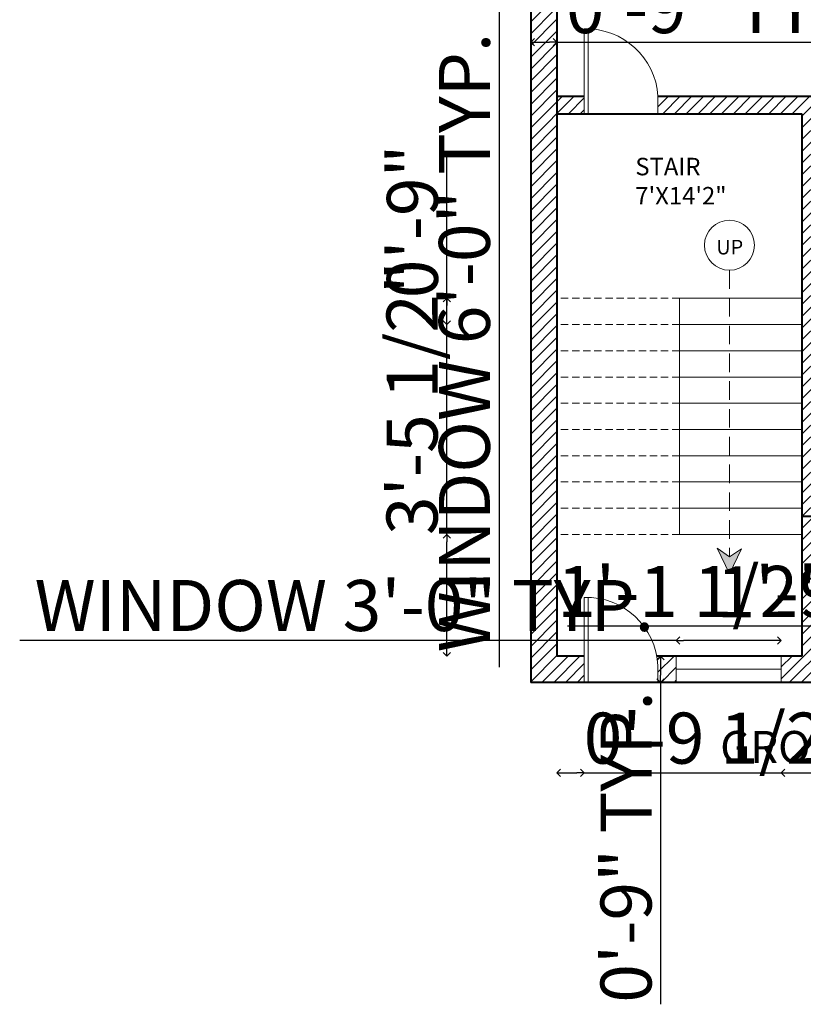
# Model space of a CAD drawing. Units: inches. Extents: x 597 to 1323, y 1833 to 2686.
# Tile 1 of 10: x 597 to 865, y 1833 to 2171. Entities that reach past the tile are written whole.
import ezdxf

# ---------------------------------------------------------------- set-up
doc = ezdxf.new("R2010")
doc.units = ezdxf.units.IN
doc.linetypes.add('DASHED', pattern=[19.05, 12.7, -6.35])
for name, color, linetype, lineweight in [('A-ANNO-DIMS', 2, 'Continuous', 18), ('A-ANNO-SYMB', 7, 'Continuous', 18), ('A-ANNO-SYMB-PATH', 7, 'DASHED', 18), ('A-ANNO-TEXT', 7, 'Continuous', 18), ('A-AREA-IDEN', 7, 'Continuous', 18), ('A-DOOR', 5, 'Continuous', 20), ('A-FLOR-STRS', 190, 'Continuous', 20), ('A-FLOR-STRS-OVHD', 190, 'DASHED', 18), ('A-GLAZ', 2, 'Continuous', 18), ('A-WALL', 7, 'Continuous', 40), ('A-WALL-PATT', 8, 'Continuous', 13)]:
    doc.layers.add(name, color=color, linetype=linetype, lineweight=lineweight)
doc.styles.get("Standard").update_dxf_attribs({"font": 'arial.ttf'})
doc.dimstyles.new('ISO-25', dxfattribs={"dimtxt": 17.5, "dimasz": 2.5, "dimexe": 0, "dimexo": 0, "dimtad": 1, "dimdec": 1, "dimlunit": 3, "dimtxsty": 'Standard', "dimblk": 'OPEN90', "dimcen": 2.5, "dimadec": 0, "dimazin": 0, "dimtfac": 1, "dimtdec": 1, "dimtmove": 0, "dimatfit": 3, "dimfxl": 0, "dimfxlon": 1, "dimarcsym": 0})

# ---------------------------------------------------------------- blocks, each defined once
blk = doc.blocks.new('DOOR-SINGLE-SWING')
for p, q in [((24, 29.15), (24, 0)), ((25.29, 0), (25.29, 29.15)), ((0, 5.64), (0, 0))]:
    blk.add_line(p, q)
blk.add_arc((24.64, 4.49), 24.67, 88.5063, 177.3274)
blk = doc.blocks.new('WINDOW-36IN')
for p, q in [((0, 0), (0, 9)), ((36, 0), (36, 9)), ((0, 4.5), (36, 4.5))]:
    blk.add_line(p, q)
blk = doc.blocks.new('_Open90')
at = {"color": 0, "linetype": 'ByBlock', "lineweight": -2}
for p, q in [((0, 0), (-1, 0)), ((-0.5, 0.5), (0, 0)), ((0, 0), (-0.5, -0.5))]:
    blk.add_line(p, q, dxfattribs=at)
blk = doc.blocks.new('*D35')
at = {"layer": 'A-ANNO-DIMS', "color": 0, "lineweight": -2, "transparency": 16777216}
for p, q in [((761.09, 2243.49), (761.09, 2176.49)), ((761.09, 2173.99), (761.09, 1948.8))]:
    blk.add_line(p, q, dxfattribs=at)
at = {"layer": 'Defpoints', "color": 0, "transparency": 16777216}
for p in [(771.89, 2245.99), (761.09, 2173.99), (771.89, 2173.99)]:
    blk.add_point(p, dxfattribs=at)
at = {"layer": 'A-ANNO-DIMS', "color": 0, "lineweight": -2, "transparency": 16777216, "xscale": 2.5, "yscale": 2.5, "zscale": 2.5}
for p, rotation in [((761.09, 2245.99), 90), ((761.09, 2173.99), 270)]:
    blk.add_blockref('_Open90', p, dxfattribs=dict(at, rotation=rotation))
at = {"layer": 'A-ANNO-DIMS', "color": 0, "transparency": 16777216, "insert": (751.41, 2060.14), "char_height": 17.5, "attachment_point": 5, "rotation": 90}
blk.add_mtext('WINDOW 6\'-0" TYP.', dxfattribs=at)
blk = doc.blocks.new('*D36')
at = {"layer": 'A-ANNO-DIMS', "color": 0, "lineweight": -2, "transparency": 16777216}
for p, q in [((774.39, 2163.19), (778.39, 2163.19)), ((780.89, 2163.19), (891.31, 2163.19))]:
    blk.add_line(p, q, dxfattribs=at)
at = {"layer": 'Defpoints', "color": 0, "transparency": 16777216}
for p in [(771.89, 2173.99), (780.89, 2173.99), (780.89, 2163.19)]:
    blk.add_point(p, dxfattribs=at)
at = {"layer": 'A-ANNO-DIMS', "color": 0, "lineweight": -2, "transparency": 16777216, "xscale": 2.5, "yscale": 2.5, "zscale": 2.5, "rotation": 180}
blk.add_blockref('_Open90', (771.89, 2163.19), dxfattribs=at)
at = {"layer": 'A-ANNO-DIMS', "color": 0, "lineweight": -2, "transparency": 16777216, "xscale": 2.5, "yscale": 2.5, "zscale": 2.5}
blk.add_blockref('_Open90', (780.89, 2163.19), dxfattribs=at)
at = {"layer": 'A-ANNO-DIMS', "color": 0, "transparency": 16777216, "insert": (837.35, 2172.75), "char_height": 17.5, "attachment_point": 5}
blk.add_mtext('0\'-9" TYP.', dxfattribs=at)
blk = doc.blocks.new('*D45')
at = {"layer": 'A-ANNO-DIMS', "color": 0, "lineweight": -2, "transparency": 16777216}
for p, q in [((821.81, 1958.01), (596.62, 1958.01)), ((855.31, 1958.01), (824.31, 1958.01))]:
    blk.add_line(p, q, dxfattribs=at)
at = {"layer": 'Defpoints', "color": 0, "transparency": 16777216}
for p in [(821.81, 1958.01), (821.81, 1952.61), (857.81, 1952.61)]:
    blk.add_point(p, dxfattribs=at)
at = {"layer": 'A-ANNO-DIMS', "color": 0, "lineweight": -2, "transparency": 16777216, "xscale": 2.5, "yscale": 2.5, "zscale": 2.5, "rotation": 180}
blk.add_blockref('_Open90', (821.81, 1958.01), dxfattribs=at)
at = {"layer": 'A-ANNO-DIMS', "color": 0, "lineweight": -2, "transparency": 16777216, "xscale": 2.5, "yscale": 2.5, "zscale": 2.5}
blk.add_blockref('_Open90', (857.81, 1958.01), dxfattribs=at)
at = {"layer": 'A-ANNO-DIMS', "color": 0, "transparency": 16777216, "insert": (707.96, 1967.7), "char_height": 17.5, "attachment_point": 5}
blk.add_mtext('WINDOW 3\'-0" TYP.', dxfattribs=at)
blk = doc.blocks.new('*D46')
at = {"layer": 'A-ANNO-DIMS', "color": 0, "lineweight": -2, "transparency": 16777216}
for p, q in [((816.41, 1950.11), (816.41, 1946.11)), ((816.41, 1943.61), (816.41, 1833.19))]:
    blk.add_line(p, q, dxfattribs=at)
at = {"layer": 'Defpoints', "color": 0, "transparency": 16777216}
for p in [(821.81, 1952.61), (816.41, 1943.61), (821.81, 1943.61)]:
    blk.add_point(p, dxfattribs=at)
at = {"layer": 'A-ANNO-DIMS', "color": 0, "lineweight": -2, "transparency": 16777216, "xscale": 2.5, "yscale": 2.5, "zscale": 2.5}
for p, rotation in [((816.41, 1952.61), 90), ((816.41, 1943.61), 270)]:
    blk.add_blockref('_Open90', p, dxfattribs=dict(at, rotation=rotation))
at = {"layer": 'A-ANNO-DIMS', "color": 0, "transparency": 16777216, "insert": (806.85, 1887.15), "char_height": 17.5, "attachment_point": 5, "rotation": 90}
blk.add_mtext('0\'-9" TYP.', dxfattribs=at)
blk = doc.blocks.new('*D55')
at = {"layer": 'A-ANNO-DIMS', "color": 0, "lineweight": -2, "transparency": 16777216}
for p, q in [((825.39, 2452.36), (862.39, 2452.36)), ((864.89, 2452.36), (915.14, 2452.36))]:
    blk.add_line(p, q, dxfattribs=at)
at = {"layer": 'Defpoints', "color": 0, "transparency": 16777216}
for p in [(864.89, 2452.36), (822.89, 2075.33), (864.89, 2075.33)]:
    blk.add_point(p, dxfattribs=at)
at = {"layer": 'A-ANNO-DIMS', "color": 0, "lineweight": -2, "transparency": 16777216, "xscale": 2.5, "yscale": 2.5, "zscale": 2.5, "rotation": 180}
blk.add_blockref('_Open90', (822.89, 2452.36), dxfattribs=at)
at = {"layer": 'A-ANNO-DIMS', "color": 0, "lineweight": -2, "transparency": 16777216, "xscale": 2.5, "yscale": 2.5, "zscale": 2.5}
blk.add_blockref('_Open90', (864.89, 2452.36), dxfattribs=at)
at = {"layer": 'A-ANNO-DIMS', "color": 0, "transparency": 16777216, "insert": (891.27, 2461.93), "char_height": 17.5, "attachment_point": 5}
blk.add_mtext('3\'-6"', dxfattribs=at)
blk = doc.blocks.new('*D56')
at = {"layer": 'A-ANNO-DIMS', "color": 0, "lineweight": -2, "transparency": 16777216}
for p, q in [((743.14, 2075.33), (743.14, 2125.6)), ((743.14, 2068.83), (743.14, 2072.83))]:
    blk.add_line(p, q, dxfattribs=at)
at = {"layer": 'Defpoints', "color": 0, "transparency": 16777216}
for p in [(743.14, 2075.33), (780.89, 2075.33), (780.89, 2066.33)]:
    blk.add_point(p, dxfattribs=at)
at = {"layer": 'A-ANNO-DIMS', "color": 0, "lineweight": -2, "transparency": 16777216, "xscale": 2.5, "yscale": 2.5, "zscale": 2.5}
for p, rotation in [((743.14, 2075.33), 90), ((743.14, 2066.33), 270)]:
    blk.add_blockref('_Open90', p, dxfattribs=dict(at, rotation=rotation))
at = {"layer": 'A-ANNO-DIMS', "color": 0, "transparency": 16777216, "insert": (733.58, 2101.72), "char_height": 17.5, "attachment_point": 5, "rotation": 90}
blk.add_mtext('0\'-9"', dxfattribs=at)
blk = doc.blocks.new('*D57')
at = {"layer": 'A-ANNO-DIMS', "color": 0, "lineweight": -2, "transparency": 16777216}
for p, q in [((743.14, 1994.33), (743.14, 2085.37)), ((743.14, 1955.11), (743.14, 1991.83))]:
    blk.add_line(p, q, dxfattribs=at)
at = {"layer": 'Defpoints', "color": 0, "transparency": 16777216}
for p in [(743.14, 1994.33), (780.89, 1994.33), (780.89, 1952.61)]:
    blk.add_point(p, dxfattribs=at)
at = {"layer": 'A-ANNO-DIMS', "color": 0, "lineweight": -2, "transparency": 16777216, "xscale": 2.5, "yscale": 2.5, "zscale": 2.5}
for p, rotation in [((743.14, 1994.33), 90), ((743.14, 1952.61), 270)]:
    blk.add_blockref('_Open90', p, dxfattribs=dict(at, rotation=rotation))
at = {"layer": 'A-ANNO-DIMS', "color": 0, "transparency": 16777216, "insert": (733.46, 2041.1), "char_height": 17.5, "attachment_point": 5, "rotation": 90}
blk.add_mtext('3\'-5 1/2"', dxfattribs=at)
blk = doc.blocks.new('*D58')
at = {"layer": 'A-ANNO-DIMS', "color": 0, "lineweight": -2, "transparency": 16777216}
for p, q in [((783.39, 1912.53), (787.76, 1912.53)), ((790.26, 1912.53), (881.3, 1912.53))]:
    blk.add_line(p, q, dxfattribs=at)
at = {"layer": 'Defpoints', "color": 0, "transparency": 16777216}
for p in [(780.89, 1952.61), (790.26, 1952.61), (790.26, 1912.53)]:
    blk.add_point(p, dxfattribs=at)
at = {"layer": 'A-ANNO-DIMS', "color": 0, "lineweight": -2, "transparency": 16777216, "xscale": 2.5, "yscale": 2.5, "zscale": 2.5, "rotation": 180}
blk.add_blockref('_Open90', (780.89, 1912.53), dxfattribs=at)
at = {"layer": 'A-ANNO-DIMS', "color": 0, "lineweight": -2, "transparency": 16777216, "xscale": 2.5, "yscale": 2.5, "zscale": 2.5}
blk.add_blockref('_Open90', (790.26, 1912.53), dxfattribs=at)
at = {"layer": 'A-ANNO-DIMS', "color": 0, "transparency": 16777216, "insert": (837.03, 1922.21), "char_height": 17.5, "attachment_point": 5}
blk.add_mtext('0\'-9 1/2"', dxfattribs=at)
blk = doc.blocks.new('*D68')
at = {"layer": 'A-ANNO-DIMS', "color": 0, "lineweight": -2, "transparency": 16777216}
for p, q in [((887.56, 1962.86), (838.94, 1962.86)), ((906.12, 1962.86), (890.06, 1962.86))]:
    blk.add_line(p, q, dxfattribs=at)
at = {"layer": 'Defpoints', "color": 0, "transparency": 16777216}
for p in [(887.56, 1991.61), (908.62, 1991.61), (887.56, 1962.86)]:
    blk.add_point(p, dxfattribs=at)
at = {"layer": 'A-ANNO-DIMS', "color": 0, "lineweight": -2, "transparency": 16777216, "xscale": 2.5, "yscale": 2.5, "zscale": 2.5, "rotation": 180}
blk.add_blockref('_Open90', (887.56, 1962.86), dxfattribs=at)
at = {"layer": 'A-ANNO-DIMS', "color": 0, "lineweight": -2, "transparency": 16777216, "xscale": 2.5, "yscale": 2.5, "zscale": 2.5}
blk.add_blockref('_Open90', (908.62, 1962.86), dxfattribs=at)
at = {"layer": 'A-ANNO-DIMS', "color": 0, "transparency": 16777216, "insert": (862, 1972.42), "char_height": 17.5, "attachment_point": 5}
blk.add_mtext('1\'-9"', dxfattribs=at)
blk = doc.blocks.new('*D77')
at = {"layer": 'A-ANNO-DIMS', "color": 0, "lineweight": -2, "transparency": 16777216}
for p, q in [((873.89, 1962.86), (784.49, 1962.86)), ((885.06, 1962.86), (876.39, 1962.86))]:
    blk.add_line(p, q, dxfattribs=at)
at = {"layer": 'Defpoints', "color": 0, "transparency": 16777216}
for p in [(873.89, 1991.61), (887.56, 1991.61), (873.89, 1962.86)]:
    blk.add_point(p, dxfattribs=at)
at = {"layer": 'A-ANNO-DIMS', "color": 0, "lineweight": -2, "transparency": 16777216, "xscale": 2.5, "yscale": 2.5, "zscale": 2.5, "rotation": 180}
blk.add_blockref('_Open90', (873.89, 1962.86), dxfattribs=at)
at = {"layer": 'A-ANNO-DIMS', "color": 0, "lineweight": -2, "transparency": 16777216, "xscale": 2.5, "yscale": 2.5, "zscale": 2.5}
blk.add_blockref('_Open90', (887.56, 1962.86), dxfattribs=at)
at = {"layer": 'A-ANNO-DIMS', "color": 0, "transparency": 16777216, "insert": (827.94, 1972.53), "char_height": 17.5, "attachment_point": 5}
blk.add_mtext('1\'-1 1/2"', dxfattribs=at)
blk = doc.blocks.new('*D78')
at = {"layer": 'A-ANNO-DIMS', "color": 0, "lineweight": -2, "transparency": 16777216}
for p, q in [((860.31, 1912.53), (871.39, 1912.53)), ((873.89, 1912.53), (922.51, 1912.53))]:
    blk.add_line(p, q, dxfattribs=at)
at = {"layer": 'Defpoints', "color": 0, "transparency": 16777216}
for p in [(857.81, 1943.61), (873.89, 1943.61), (873.89, 1912.53)]:
    blk.add_point(p, dxfattribs=at)
at = {"layer": 'A-ANNO-DIMS', "color": 0, "lineweight": -2, "transparency": 16777216, "xscale": 2.5, "yscale": 2.5, "zscale": 2.5, "rotation": 180}
blk.add_blockref('_Open90', (857.81, 1912.53), dxfattribs=at)
at = {"layer": 'A-ANNO-DIMS', "color": 0, "lineweight": -2, "transparency": 16777216, "xscale": 2.5, "yscale": 2.5, "zscale": 2.5}
blk.add_blockref('_Open90', (873.89, 1912.53), dxfattribs=at)
at = {"layer": 'A-ANNO-DIMS', "color": 0, "transparency": 16777216, "insert": (899.45, 1921.95), "char_height": 17.5, "attachment_point": 5}
blk.add_mtext('1\'-4"', dxfattribs=at)

msp = doc.modelspace()

# ---------------------------------------------------------------- hatches: boundary and pattern name
at = {"layer": 'A-ANNO-SYMB'}
h = msp.add_hatch(color=256, dxfattribs=at)
h.dxf.hatch_style = 1
h.paths.add_polyline_path([(844.16, 1989.4), (840.06, 1986.69), (835.79, 1989.64), (840.03, 1980.79)])
at = {"layer": 'A-WALL-PATT'}
h = msp.add_hatch(dxfattribs=at)
h.set_pattern_fill('ANSI31', color=256, scale=0.9)
h.paths.add_polyline_path([(927.93, 2423.61), (771.89, 2423.61), (771.89, 2371.61), (780.89, 2371.61), (780.89, 2414.61), (918.89, 2414.61), (927.93, 2414.61)])
h.paths.add_polyline_path([(1107.89, 2423.61), (1074.89, 2423.61), (1074.89, 2414.61), (1098.89, 2414.61), (1098.89, 2382.26), (1107.89, 2382.26)])
h.paths.add_polyline_path([(1002.89, 2423.61), (963.93, 2423.61), (963.93, 2414.61), (978.89, 2414.61), (1002.89, 2414.61)])
h.paths.add_polyline_path([(918.89, 2414.61), (912.89, 2414.61), (912.89, 2270.61), (906.2, 2270.61), (906.2, 2264.61), (918.89, 2264.61), (918.89, 2318.61), (928.09, 2318.61), (928.09, 2324.61), (918.89, 2324.61)])
h.paths.add_polyline_path([(780.89, 2299.61), (771.89, 2299.61), (771.89, 2245.99), (780.89, 2245.99)])
h.paths.add_polyline_path([(780.89, 2173.99), (771.89, 2173.99), (771.89, 1943.61), (790.26, 1943.61), (790.26, 1952.61), (780.89, 1952.61)])
h.paths.add_polyline_path([(873.89, 1991.61), (887.56, 1991.61), (887.56, 2000.61), (864.89, 2000.61), (864.89, 1952.61), (857.81, 1952.61), (857.81, 1943.61), (873.89, 1943.61)])
h.paths.add_polyline_path([(979.81, 2000.61), (908.62, 2000.61), (908.62, 1991.61), (979.81, 1991.61)])
h.paths.add_polyline_path([(931.89, 2138.61), (938.68, 2138.61), (938.68, 2144.61), (925.89, 2144.61), (925.89, 2000.61), (931.89, 2000.61)])
h.paths.add_polyline_path([(870.89, 2084.61), (874.89, 2084.61), (874.89, 2090.61), (870.89, 2090.61), (870.89, 2144.61), (815.52, 2144.61), (815.52, 2138.61), (864.89, 2138.61), (864.89, 2000.61), (870.89, 2000.61)])
h.paths.add_polyline_path([(925.89, 2090.61), (900.18, 2090.61), (900.18, 2084.61), (925.89, 2084.61)])
h.paths.add_polyline_path([(1107.89, 2051.2), (1098.89, 2051.2), (1098.89, 2000.61), (1047.65, 2000.61), (1047.65, 1991.61), (1107.89, 1991.61)])
h.paths.add_polyline_path([(1107.89, 2181.44), (1098.89, 2181.44), (1098.89, 2109.76), (1107.89, 2109.76)])
h.paths.add_polyline_path([(1098.89, 2144.61), (978.89, 2144.61), (978.89, 2157.94), (972.89, 2157.94), (972.89, 2144.61), (963.97, 2144.61), (963.97, 2138.61), (1098.89, 2138.61)])
h.paths.add_polyline_path([(1107.89, 2310.26), (1098.89, 2310.26), (1098.89, 2227.53), (1107.89, 2227.53)])
h.paths.add_polyline_path([(1098.89, 2270.61), (978.89, 2270.61), (978.89, 2276), (972.89, 2276), (972.89, 2183.23), (978.89, 2183.23), (978.89, 2264.61), (1098.89, 2264.61)])
h.paths.add_polyline_path([(880.92, 2270.61), (780.89, 2270.61), (780.89, 2264.61), (880.92, 2264.61)])
h.paths.add_polyline_path([(978.89, 2414.61), (972.89, 2414.61), (972.89, 2324.61), (961.07, 2324.61), (961.07, 2318.61), (972.89, 2318.61), (972.89, 2301.29), (978.89, 2301.29)])
h.paths.add_polyline_path([(790.26, 2144.61), (780.89, 2144.61), (780.89, 2138.61), (790.26, 2138.61)], flags=17)
h = msp.add_hatch(dxfattribs=at)
h.set_pattern_fill('ANSI31', color=256)
h.paths.add_polyline_path([(821.81, 1952.61), (815.15, 1952.61, -0.034288), (815.54, 1949.25), (815.54, 1943.61), (821.81, 1943.61)])

# ---------------------------------------------------------------- linework, layer by layer
at = {"layer": 'A-ANNO-SYMB'}
for p, q in [((840.06, 1986.69), (835.79, 1989.64)), ((835.79, 1989.64), (840.03, 1980.79)), ((840.03, 1980.79), (844.16, 1989.4)), ((840.06, 1986.69), (844.16, 1989.4))]:
    msp.add_line(p, q, dxfattribs=at)
msp.add_circle((840.06, 2093.53), 8.57, dxfattribs=at)
at = {"layer": 'A-ANNO-SYMB-PATH', "ltscale": 0.5}
msp.add_line((840.06, 2084.96), (840.06, 1986.69), dxfattribs=at)
at = {"layer": 'A-DOOR'}
for p, q in [((790.26, 2138.61), (790.26, 2167.76)), ((790.26, 2138.61), (790.26, 2167.76)), ((791.54, 2167.76), (791.54, 2138.61)), ((791.54, 2167.76), (791.54, 2138.61)), ((815.52, 2144.61), (815.52, 2138.61)), ((790.26, 1943.61), (790.26, 1972.76)), ((791.54, 1972.76), (791.54, 1943.61))]:
    msp.add_line(p, q, dxfattribs=at)
for centre, start in [((790.9, 2143.1), 3.5034), ((790.9, 1948.1), 2.6726)]:
    msp.add_arc(centre, 24.67, start, 91.4937, dxfattribs=at)
at = {"layer": 'A-FLOR-STRS'}
for p, q in [((822.89, 2075.33), (822.89, 1994.33)), ((864.89, 2075.33), (822.89, 2075.33)), ((864.89, 2066.33), (822.89, 2066.33)), ((864.89, 2057.33), (822.89, 2057.33)), ((864.89, 2048.33), (822.89, 2048.33)), ((864.89, 2039.33), (822.89, 2039.33)), ((864.89, 2030.33), (822.89, 2030.33)), ((864.89, 2021.33), (822.89, 2021.33)), ((864.89, 2012.33), (822.89, 2012.33)), ((864.89, 2003.33), (822.89, 2003.33)), ((864.89, 1994.33), (822.89, 1994.33))]:
    msp.add_line(p, q, dxfattribs=at)
at = {"layer": 'A-FLOR-STRS-OVHD', "ltscale": 0.2}
for p, q in [((822.89, 2075.33), (780.89, 2075.33)), ((822.89, 2066.33), (780.89, 2066.33)), ((822.89, 2057.33), (780.89, 2057.33)), ((822.89, 2048.33), (780.89, 2048.33)), ((822.89, 2039.33), (780.89, 2039.33)), ((822.89, 2030.33), (780.89, 2030.33)), ((822.89, 2021.33), (780.89, 2021.33)), ((822.89, 2012.33), (780.89, 2012.33)), ((822.89, 2003.33), (780.89, 2003.33)), ((822.89, 1994.33), (780.89, 1994.33))]:
    msp.add_line(p, q, dxfattribs=at)
at = {"layer": 'A-WALL'}
for p, q in [((771.89, 2423.61), (771.89, 1943.61)), ((780.89, 2414.61), (780.89, 1952.61)), ((780.89, 2144.61), (790.26, 2144.61)), ((815.52, 2144.61), (870.89, 2144.61)), ((780.89, 2138.61), (864.89, 2138.61)), ((864.89, 2138.61), (864.89, 1952.61)), ((864.89, 2000.61), (1098.89, 2000.61)), ((790.26, 1952.61), (780.89, 1952.61)), ((864.89, 1952.61), (815.15, 1952.61)), ((1107.89, 1943.61), (771.89, 1943.61))]:
    msp.add_line(p, q, dxfattribs=at)

# ---------------------------------------------------------------- block references
at = {"layer": 'A-DOOR', "extrusion": (0, 0, -1), "zscale": -1}
msp.add_blockref('DOOR-SINGLE-SWING', (-815.54, 1943.61), dxfattribs=at)
at = {"layer": 'A-GLAZ', "rotation": 180}
msp.add_blockref('WINDOW-36IN', (857.81, 1952.61), dxfattribs=at)

# ---------------------------------------------------------------- texts
at = {"layer": 'A-ANNO-TEXT', "attachment_point": 1}
for s, width, insert, char_height in [('UP', 10.478, (835.53, 2095.38), 5), ('GROUND RLOOR PLAN', 624.2346, (836.87, 1926.94), 11)]:
    msp.add_mtext_dynamic_manual_height_columns(s, width=width, gutter_width=12.5, heights=[0], dxfattribs=dict(at, insert=insert, char_height=char_height))
at = {"layer": 'A-AREA-IDEN', "insert": (807.77, 2123.51), "char_height": 6, "attachment_point": 1}
msp.add_mtext_dynamic_manual_height_columns('STAIR\\P7\'X14\'2"', width=54.7527, gutter_width=12.5, heights=[0], dxfattribs=at)

# ---------------------------------------------------------------- dimensions: what is measured, and where the dimension line sits
at = {"layer": 'A-ANNO-DIMS'}
for base, p1, p2, picture, middle in [((864.89, 2452.36), (822.89, 2075.33), (864.89, 2075.33), '*D55', (891.27, 2461.93)), ((790.26, 1912.53), (780.89, 1952.61), (790.26, 1952.61), '*D58', (837.03, 1922.21)), ((873.89, 1912.53), (857.81, 1943.61), (873.89, 1943.61), '*D78', (899.45, 1921.95))]:
    dim = msp.add_linear_dim(base=base, p1=p1, p2=p2, dimstyle='ISO-25', override={"dimdec": 1, "dimlfac": 1, "dimrnd": 0, "dimzin": 1, "dimdsep": 46, "dimlunit": 4, "dimfrac": 2}, dxfattribs=at)
    dim.commit()
    dim.dimension.update_dxf_attribs({"geometry": picture, "text_midpoint": middle})
for base, p1, p2, angle, text, picture, middle in [((761.09, 2173.99), (771.89, 2245.99), (771.89, 2173.99), 270, 'WINDOW <> TYP.', '*D35', (751.41, 2060.14)), ((821.81, 1958.01), (857.81, 1952.61), (821.81, 1952.61), 180, 'WINDOW <> TYP.', '*D45', (707.96, 1967.7)), ((816.41, 1943.61), (821.81, 1952.61), (821.81, 1943.61), 270, '<> TYP.', '*D46', (806.85, 1887.15))]:
    dim = msp.add_linear_dim(base=base, p1=p1, p2=p2, angle=angle, text=text, dimstyle='ISO-25', override={"dimdec": 1, "dimlfac": 1, "dimrnd": 0, "dimzin": 1, "dimdsep": 46, "dimlunit": 4, "dimfrac": 2}, dxfattribs=at)
    dim.commit()
    dim.dimension.update_dxf_attribs({"geometry": picture, "text_midpoint": middle})
dim = msp.add_linear_dim(base=(780.89, 2163.19), p1=(771.89, 2173.99), p2=(780.89, 2173.99), text='<> TYP.', dimstyle='ISO-25', override={"dimdec": 1, "dimlfac": 1, "dimrnd": 0, "dimzin": 1, "dimdsep": 46, "dimlunit": 4, "dimfrac": 2}, dxfattribs=at)
dim.commit()
dim.dimension.update_dxf_attribs({"geometry": '*D36', "text_midpoint": (837.35, 2172.75)})
for base, p1, p2, angle, picture, middle in [((743.14, 2075.33), (780.89, 2066.33), (780.89, 2075.33), 90, '*D56', (733.58, 2101.72)), ((743.14, 1994.33), (780.89, 1952.61), (780.89, 1994.33), 90, '*D57', (733.46, 2041.1)), ((873.89, 1962.86), (887.56, 1991.61), (873.89, 1991.61), 180, '*D77', (827.94, 1972.53)), ((887.56, 1962.86), (908.62, 1991.61), (887.56, 1991.61), 180, '*D68', (862, 1972.42))]:
    dim = msp.add_linear_dim(base=base, p1=p1, p2=p2, angle=angle, dimstyle='ISO-25', override={"dimdec": 1, "dimlfac": 1, "dimrnd": 0, "dimzin": 1, "dimdsep": 46, "dimlunit": 4, "dimfrac": 2}, dxfattribs=at)
    dim.commit()
    dim.dimension.update_dxf_attribs({"geometry": picture, "text_midpoint": middle})

doc.saveas('drawing.dxf')
